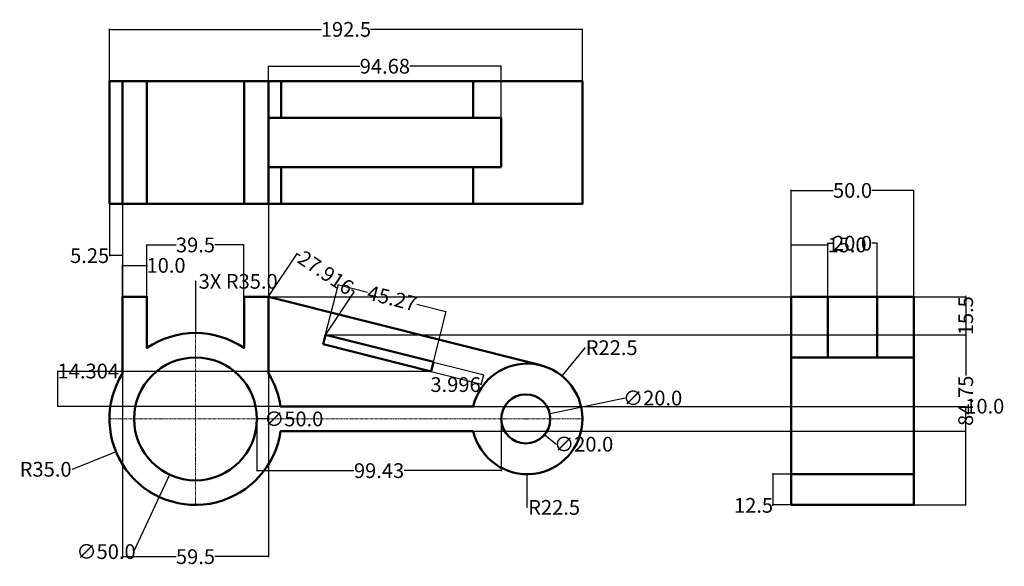
# Model space of a CAD drawing. Units: millimetres. Extents: x -7 to 393, y 19 to 241.
import ezdxf

# ---------------------------------------------------------------- set-up
doc = ezdxf.new("R2010")
doc.units = ezdxf.units.MM
doc.header["$MEASUREMENT"] = 0
doc.linetypes.add('CENTER', pattern=[2, 1.25, -0.25, 0.25, -0.25])
for name, color, linetype, lineweight in [('M-CNTR', 4, 'CENTER', 18), ('M-DIMS', 2, 'Continuous', 25), ('M-OUTL', 7, 'Continuous', 50)]:
    doc.layers.add(name, color=color, linetype=linetype, lineweight=lineweight)
doc.styles.get("Standard").update_dxf_attribs({"font": 'arial.ttf'})
doc.dimstyles.get("Standard").update_dxf_attribs({"dimtxt": 6, "dimasz": 0.18, "dimexe": 0.18, "dimexo": 0.0625, "dimgap": 0.09, "dimtad": 0, "dimtoh": 1, "dimdec": 1, "dimzin": 0, "dimdsep": 46, "dimtxsty": 'Standard', "dimcen": 0.09, "dimadec": 0, "dimazin": 0, "dimtfac": 1, "dimtdec": 1, "dimtofl": 0, "dimtmove": 0, "dimatfit": 3, "dimfxl": 1, "dimtolj": 1, "dimtzin": 0, "dimarcsym": 0})

# ---------------------------------------------------------------- blocks, each defined once
blk = doc.blocks.new('*D1')
at = {"layer": 'Defpoints', "color": 0, "transparency": 16777216}
for p in [(356.5, 171.5), (306.5, 128.25), (356.5, 128.25)]:
    blk.add_point(p, dxfattribs=at)
at = {"layer": 'M-DIMS', "color": 0, "lineweight": -2, "transparency": 16777216}
for p, q in [((306.5, 128.31), (306.5, 171.68)), ((306.68, 171.5), (323.63, 171.5)), ((356.32, 171.5), (339.37, 171.5)), ((356.5, 128.31), (356.5, 171.68))]:
    blk.add_line(p, q, dxfattribs=at)
at = {"layer": 'M-DIMS', "color": 0, "transparency": 16777216}
for points in [[(306.68, 171.53), (306.68, 171.47), (306.5, 171.5)], [(356.32, 171.53), (356.32, 171.47), (356.5, 171.5)]]:
    blk.add_solid(points, dxfattribs=at)
at = {"layer": 'M-DIMS', "color": 0, "transparency": 16777216, "insert": (331.5, 171.5), "char_height": 6, "attachment_point": 5}
blk.add_mtext('\\A1;50.0', dxfattribs=at)
blk = doc.blocks.new('*D2')
at = {"layer": 'Defpoints', "color": 0, "transparency": 16777216}
for p in [(341.5, 150), (321.5, 128.25), (341.5, 128.25)]:
    blk.add_point(p, dxfattribs=at)
at = {"layer": 'M-DIMS', "color": 0, "lineweight": -2, "transparency": 16777216}
for p, q in [((321.5, 128.31), (321.5, 150.18)), ((321.68, 150), (323.58, 150)), ((341.32, 150), (339.42, 150)), ((341.5, 128.31), (341.5, 150.18))]:
    blk.add_line(p, q, dxfattribs=at)
at = {"layer": 'M-DIMS', "color": 0, "transparency": 16777216}
for points in [[(321.68, 150.03), (321.68, 149.97), (321.5, 150)], [(341.32, 150.03), (341.32, 149.97), (341.5, 150)]]:
    blk.add_solid(points, dxfattribs=at)
at = {"layer": 'M-DIMS', "color": 0, "transparency": 16777216, "insert": (331.5, 150), "char_height": 6, "attachment_point": 5}
blk.add_mtext('\\A1;20.0', dxfattribs=at)
blk = doc.blocks.new('*D3')
at = {"layer": 'Defpoints', "color": 0, "transparency": 16777216}
for p in [(306.5, 56), (299, 43.5), (306.5, 43.5)]:
    blk.add_point(p, dxfattribs=at)
at = {"layer": 'M-DIMS', "color": 0, "lineweight": -2, "transparency": 16777216}
for p, q in [((306.44, 56), (298.82, 56)), ((299, 55.82), (299, 43.68)), ((306.44, 43.5), (298.82, 43.5)), ((299, 43.32), (298.82, 43.32)), ((299, 43.5), (299, 43.32))]:
    blk.add_line(p, q, dxfattribs=at)
at = {"layer": 'M-DIMS', "color": 0, "transparency": 16777216}
for points in [[(298.97, 55.82), (299.03, 55.82), (299, 56)], [(298.97, 43.68), (299.03, 43.68), (299, 43.5)]]:
    blk.add_solid(points, dxfattribs=at)
at = {"layer": 'M-DIMS', "color": 0, "transparency": 16777216, "insert": (291.2, 43.32), "char_height": 6, "attachment_point": 5}
blk.add_mtext('\\A1;12.5', dxfattribs=at)
blk = doc.blocks.new('*D4')
at = {"layer": 'Defpoints', "color": 0, "transparency": 16777216}
for p in [(213.21, 96), (199.07, 78.5)]:
    blk.add_point(p, dxfattribs=at)
at = {"layer": 'M-DIMS', "color": 0, "lineweight": -2, "transparency": 16777216}
for p, q in [((222.5, 107.5), (213.32, 96.14)), ((222.68, 107.5), (222.5, 107.5)), ((198.98, 78.5), (199.16, 78.5)), ((199.07, 78.41), (199.07, 78.59))]:
    blk.add_line(p, q, dxfattribs=at)
at = {"layer": 'M-DIMS', "color": 0, "transparency": 16777216}
blk.add_solid([(213.3, 96.16), (213.35, 96.12), (213.21, 96)], dxfattribs=at)
at = {"layer": 'M-DIMS', "color": 0, "transparency": 16777216, "insert": (233.46, 107.5), "char_height": 6, "attachment_point": 5}
blk.add_mtext('\\A1;R22.5', dxfattribs=at)
blk = doc.blocks.new('*D5')
at = {"layer": 'Defpoints', "color": 0, "transparency": 16777216}
for p in [(208.29, 80.55), (188.71, 76.45)]:
    blk.add_point(p, dxfattribs=at)
at = {"layer": 'M-DIMS', "color": 0, "lineweight": -2, "transparency": 16777216}
for p, q in [((239, 87), (208.46, 80.59)), ((198.41, 78.5), (198.59, 78.5)), ((198.5, 78.41), (198.5, 78.59))]:
    blk.add_line(p, q, dxfattribs=at)
at = {"layer": 'M-DIMS', "color": 0, "transparency": 16777216}
blk.add_solid([(208.46, 80.62), (208.47, 80.56), (208.29, 80.55)], dxfattribs=at)
at = {"layer": 'M-DIMS', "color": 0, "transparency": 16777216, "insert": (250.14, 87), "char_height": 6, "attachment_point": 5}
blk.add_mtext('\\A1;∅20.0', dxfattribs=at)
blk = doc.blocks.new('*D6')
at = {"layer": 'Defpoints', "color": 0, "transparency": 16777216}
for p in [(44.32, 141), (34.32, 128.25), (44.32, 128.25)]:
    blk.add_point(p, dxfattribs=at)
at = {"layer": 'M-DIMS', "color": 0, "lineweight": -2, "transparency": 16777216}
for p, q in [((34.32, 128.31), (34.32, 141.18)), ((34.5, 141), (44.14, 141)), ((44.32, 128.31), (44.32, 141.18)), ((44.32, 141), (44.5, 141))]:
    blk.add_line(p, q, dxfattribs=at)
at = {"layer": 'M-DIMS', "color": 0, "transparency": 16777216}
for points in [[(34.5, 141.03), (34.5, 140.97), (34.32, 141)], [(44.14, 141.03), (44.14, 140.97), (44.32, 141)]]:
    blk.add_solid(points, dxfattribs=at)
at = {"layer": 'M-DIMS', "color": 0, "transparency": 16777216, "insert": (52.09, 141), "char_height": 6, "attachment_point": 5}
blk.add_mtext('\\A1;10.0', dxfattribs=at)
blk = doc.blocks.new('*D7')
at = {"layer": 'Defpoints', "color": 0, "transparency": 16777216}
for p in [(64.07, 78.5), (31.68, 65.24)]:
    blk.add_point(p, dxfattribs=at)
at = {"layer": 'M-DIMS', "color": 0, "lineweight": -2, "transparency": 16777216}
for p, q in [((63.98, 78.5), (64.16, 78.5)), ((64.07, 78.41), (64.07, 78.59)), ((14, 58), (31.51, 65.17)), ((13.82, 58), (14, 58))]:
    blk.add_line(p, q, dxfattribs=at)
at = {"layer": 'M-DIMS', "color": 0, "transparency": 16777216}
blk.add_solid([(31.5, 65.2), (31.53, 65.14), (31.68, 65.24)], dxfattribs=at)
at = {"layer": 'M-DIMS', "color": 0, "transparency": 16777216, "insert": (3.08, 58), "char_height": 6, "attachment_point": 5}
blk.add_mtext('\\A1;R35.0', dxfattribs=at)
blk = doc.blocks.new('*D8')
at = {"layer": 'Defpoints', "color": 0, "transparency": 16777216}
for p in [(74.6, 101.18), (53.54, 55.82)]:
    blk.add_point(p, dxfattribs=at)
at = {"layer": 'M-DIMS', "color": 0, "lineweight": -2, "transparency": 16777216}
for p, q in [((63.98, 78.5), (64.16, 78.5)), ((64.07, 78.41), (64.07, 78.59)), ((39, 24.5), (53.47, 55.66)), ((38.82, 24.5), (39, 24.5))]:
    blk.add_line(p, q, dxfattribs=at)
at = {"layer": 'M-DIMS', "color": 0, "transparency": 16777216}
blk.add_solid([(53.44, 55.67), (53.5, 55.65), (53.54, 55.82)], dxfattribs=at)
at = {"layer": 'M-DIMS', "color": 0, "transparency": 16777216, "insert": (27.68, 24.5), "char_height": 6, "attachment_point": 5}
blk.add_mtext('\\A1;∅50.0', dxfattribs=at)
blk = doc.blocks.new('*D9')
at = {"layer": 'Defpoints', "color": 0, "transparency": 16777216}
for p in [(221.57, 237.05), (29.07, 216), (221.57, 216)]:
    blk.add_point(p, dxfattribs=at)
at = {"layer": 'M-DIMS', "color": 0, "lineweight": -2, "transparency": 16777216}
for p, q in [((29.07, 216.06), (29.07, 237.23)), ((29.25, 237.05), (115.37, 237.05)), ((221.39, 237.05), (135.28, 237.05)), ((221.57, 216.06), (221.57, 237.23))]:
    blk.add_line(p, q, dxfattribs=at)
at = {"layer": 'M-DIMS', "color": 0, "transparency": 16777216}
for points in [[(29.25, 237.08), (29.25, 237.02), (29.07, 237.05)], [(221.39, 237.08), (221.39, 237.02), (221.57, 237.05)]]:
    blk.add_solid(points, dxfattribs=at)
at = {"layer": 'M-DIMS', "color": 0, "transparency": 16777216, "insert": (125.32, 237.05), "char_height": 6, "attachment_point": 5}
blk.add_mtext('\\A1;192.5', dxfattribs=at)
blk = doc.blocks.new('*D10')
at = {"layer": 'Defpoints', "color": 0, "transparency": 16777216}
for p in [(356.5, 128.25), (377.55, 128.25), (356.5, 43.5)]:
    blk.add_point(p, dxfattribs=at)
at = {"layer": 'M-DIMS', "color": 0, "lineweight": -2, "transparency": 16777216}
for p, q in [((356.56, 128.25), (377.73, 128.25)), ((377.55, 128.07), (377.55, 96.12)), ((377.55, 43.68), (377.55, 75.63)), ((356.56, 43.5), (377.73, 43.5))]:
    blk.add_line(p, q, dxfattribs=at)
at = {"layer": 'M-DIMS', "color": 0, "transparency": 16777216}
for points in [[(377.52, 128.07), (377.58, 128.07), (377.55, 128.25)], [(377.52, 43.68), (377.58, 43.68), (377.55, 43.5)]]:
    blk.add_solid(points, dxfattribs=at)
at = {"layer": 'M-DIMS', "color": 0, "transparency": 16777216, "insert": (377.55, 85.87), "char_height": 6, "attachment_point": 5, "rotation": 90}
blk.add_mtext('\\A1;84.75', dxfattribs=at)
blk = doc.blocks.new('*D11')
at = {"layer": 'Defpoints', "color": 0, "transparency": 16777216}
for p in [(89.07, 78.5), (188.5, 78.5), (89.07, 57.45)]:
    blk.add_point(p, dxfattribs=at)
at = {"layer": 'M-DIMS', "color": 0, "lineweight": -2, "transparency": 16777216}
for p, q in [((89.07, 78.44), (89.07, 57.27)), ((188.5, 78.44), (188.5, 57.27)), ((89.25, 57.45), (128.57, 57.45)), ((188.32, 57.45), (149, 57.45))]:
    blk.add_line(p, q, dxfattribs=at)
at = {"layer": 'M-DIMS', "color": 0, "transparency": 16777216}
for points in [[(89.25, 57.48), (89.25, 57.42), (89.07, 57.45)], [(188.32, 57.48), (188.32, 57.42), (188.5, 57.45)]]:
    blk.add_solid(points, dxfattribs=at)
at = {"layer": 'M-DIMS', "color": 0, "transparency": 16777216, "insert": (138.79, 57.45), "char_height": 6, "attachment_point": 5}
blk.add_mtext('\\A1;99.43', dxfattribs=at)
blk = doc.blocks.new('*D12')
at = {"layer": 'Defpoints', "color": 0, "transparency": 16777216}
for p in [(98.712775, 83.5), (377.55, 83.5), (98.712775, 73.5)]:
    blk.add_point(p, dxfattribs=at)
at = {"layer": 'M-DIMS', "color": 0, "lineweight": -2, "transparency": 16777216}
for p, q in [((98.775275, 83.5), (377.73, 83.5)), ((377.55, 83.5), (377.55, 83.68)), ((377.55, 83.68), (377.73, 83.68)), ((377.55, 73.68), (377.55, 83.32)), ((98.775275, 73.5), (377.73, 73.5))]:
    blk.add_line(p, q, dxfattribs=at)
at = {"layer": 'M-DIMS', "color": 0, "transparency": 16777216}
for points in [[(377.52, 83.32), (377.58, 83.32), (377.55, 83.5)], [(377.52, 73.68), (377.58, 73.68), (377.55, 73.5)]]:
    blk.add_solid(points, dxfattribs=at)
at = {"layer": 'M-DIMS', "color": 0, "transparency": 16777216, "insert": (385.32, 83.68), "char_height": 6, "attachment_point": 5}
blk.add_mtext('\\A1;10.0', dxfattribs=at)
blk = doc.blocks.new('*D13')
at = {"layer": 'Defpoints', "color": 0, "transparency": 16777216}
for p in [(34.32, 166), (93.82, 166), (93.82, 22.45)]:
    blk.add_point(p, dxfattribs=at)
at = {"layer": 'M-DIMS', "color": 0, "lineweight": -2, "transparency": 16777216}
for p, q in [((34.32, 165.94), (34.32, 22.27)), ((93.82, 165.94), (93.82, 22.27)), ((34.5, 22.45), (56.17, 22.45)), ((93.64, 22.45), (71.98, 22.45))]:
    blk.add_line(p, q, dxfattribs=at)
at = {"layer": 'M-DIMS', "color": 0, "transparency": 16777216}
for points in [[(34.5, 22.48), (34.5, 22.42), (34.32, 22.45)], [(93.64, 22.48), (93.64, 22.42), (93.82, 22.45)]]:
    blk.add_solid(points, dxfattribs=at)
at = {"layer": 'M-DIMS', "color": 0, "transparency": 16777216, "insert": (64.07, 22.45), "char_height": 6, "attachment_point": 5}
blk.add_mtext('\\A1;59.5', dxfattribs=at)
blk = doc.blocks.new('*D14')
at = {"layer": 'Defpoints', "color": 0, "transparency": 16777216}
for p in [(166.08, 122.09), (117.04, 112.75), (160.93, 101.68)]:
    blk.add_point(p, dxfattribs=at)
at = {"layer": 'M-DIMS', "color": 0, "lineweight": -2, "transparency": 16777216}
for p, q in [((117.05, 112.81), (122.23, 133.34)), ((122.36, 133.12), (134.11, 130.15)), ((165.91, 122.13), (154.16, 125.1)), ((160.95, 101.74), (166.13, 122.26))]:
    blk.add_line(p, q, dxfattribs=at)
at = {"layer": 'M-DIMS', "color": 0, "transparency": 16777216}
for points in [[(122.37, 133.15), (122.35, 133.09), (122.19, 133.16)], [(165.92, 122.16), (165.9, 122.1), (166.08, 122.09)]]:
    blk.add_solid(points, dxfattribs=at)
at = {"layer": 'M-DIMS', "color": 0, "transparency": 16777216, "insert": (144.13, 127.63), "char_height": 6, "attachment_point": 5, "rotation": 345.8445}
blk.add_mtext('\\A1;45.27', dxfattribs=at)
blk = doc.blocks.new('*D15')
at = {"layer": 'Defpoints', "color": 0, "transparency": 16777216}
for p in [(160.93, 101.68), (159.96, 97.8), (180.37, 92.66)]:
    blk.add_point(p, dxfattribs=at)
at = {"layer": 'M-DIMS', "color": 0, "lineweight": -2, "transparency": 16777216}
for p, q in [((160.99, 101.66), (181.52, 96.49)), ((160.02, 97.79), (180.54, 92.61)), ((181.3, 96.36), (180.41, 92.83)), ((180.32, 92.48), (180.14, 92.48)), ((180.37, 92.66), (180.32, 92.48))]:
    blk.add_line(p, q, dxfattribs=at)
at = {"layer": 'M-DIMS', "color": 0, "transparency": 16777216}
for points in [[(181.27, 96.36), (181.33, 96.35), (181.35, 96.53)], [(180.38, 92.84), (180.44, 92.82), (180.37, 92.66)]]:
    blk.add_solid(points, dxfattribs=at)
at = {"layer": 'M-DIMS', "color": 0, "transparency": 16777216, "insert": (169.93, 92.48), "char_height": 6, "attachment_point": 5}
blk.add_mtext('\\A1;3.996', dxfattribs=at)
blk = doc.blocks.new('*D16')
at = {"layer": 'Defpoints', "color": 0, "transparency": 16777216}
for p in [(93.82, 128.25), (117.04, 112.75), (377.55, 112.75)]:
    blk.add_point(p, dxfattribs=at)
at = {"layer": 'M-DIMS', "color": 0, "lineweight": -2, "transparency": 16777216}
for p, q in [((93.88, 128.25), (377.73, 128.25)), ((377.55, 128.43), (377.55, 128.61)), ((117.1, 112.75), (377.73, 112.75)), ((377.55, 112.57), (377.55, 112.39))]:
    blk.add_line(p, q, dxfattribs=at)
at = {"layer": 'M-DIMS', "color": 0, "transparency": 16777216}
for points in [[(377.52, 128.43), (377.58, 128.43), (377.55, 128.25)], [(377.52, 112.57), (377.58, 112.57), (377.55, 112.75)]]:
    blk.add_solid(points, dxfattribs=at)
at = {"layer": 'M-DIMS', "color": 0, "transparency": 16777216, "insert": (377.55, 120.5), "char_height": 6, "attachment_point": 5, "rotation": 90}
blk.add_mtext('\\A1;15.5', dxfattribs=at)
blk = doc.blocks.new('*D17')
at = {"layer": 'Defpoints', "color": 0, "transparency": 16777216}
for p in [(188.5, 222.05), (93.82, 201), (188.5, 201)]:
    blk.add_point(p, dxfattribs=at)
at = {"layer": 'M-DIMS', "color": 0, "lineweight": -2, "transparency": 16777216}
for p, q in [((93.82, 201.06), (93.82, 222.23)), ((94, 222.05), (130.94, 222.05)), ((188.32, 222.05), (151.38, 222.05)), ((188.5, 201.06), (188.5, 222.23))]:
    blk.add_line(p, q, dxfattribs=at)
at = {"layer": 'M-DIMS', "color": 0, "transparency": 16777216}
for points in [[(94, 222.08), (94, 222.02), (93.82, 222.05)], [(188.32, 222.08), (188.32, 222.02), (188.5, 222.05)]]:
    blk.add_solid(points, dxfattribs=at)
at = {"layer": 'M-DIMS', "color": 0, "transparency": 16777216, "insert": (141.16, 222.05), "char_height": 6, "attachment_point": 5}
blk.add_mtext('\\A1;94.68', dxfattribs=at)
blk = doc.blocks.new('*D18')
at = {"layer": 'Defpoints', "color": 0, "transparency": 16777216}
for p in [(93.82, 128.25), (128.73, 130.26), (117.04, 112.75)]:
    blk.add_point(p, dxfattribs=at)
at = {"layer": 'M-DIMS', "color": 0, "lineweight": -2, "transparency": 16777216}
for p, q in [((93.86, 128.3), (105.61, 145.91)), ((105.66, 145.66), (106.64, 145)), ((117.07, 112.8), (128.83, 130.41)), ((128.58, 130.36), (127.59, 131.01))]:
    blk.add_line(p, q, dxfattribs=at)
at = {"layer": 'M-DIMS', "color": 0, "transparency": 16777216}
for points in [[(105.68, 145.68), (105.64, 145.63), (105.51, 145.76)], [(128.59, 130.38), (128.56, 130.33), (128.73, 130.26)]]:
    blk.add_solid(points, dxfattribs=at)
at = {"layer": 'M-DIMS', "color": 0, "transparency": 16777216, "insert": (117.12, 138.01), "char_height": 6, "attachment_point": 5, "rotation": 326.2729}
blk.add_mtext('\\A1;27.916', dxfattribs=at)
blk = doc.blocks.new('*D19')
at = {"layer": 'Defpoints', "color": 0, "transparency": 16777216}
for p in [(29.07, 166), (34.32, 166), (29.07, 144.95)]:
    blk.add_point(p, dxfattribs=at)
at = {"layer": 'M-DIMS', "color": 0, "lineweight": -2, "transparency": 16777216}
for p, q in [((29.07, 165.94), (29.07, 144.77)), ((34.32, 165.94), (34.32, 144.77)), ((29.07, 144.95), (28.89, 144.95)), ((34.14, 144.95), (29.25, 144.95))]:
    blk.add_line(p, q, dxfattribs=at)
at = {"layer": 'M-DIMS', "color": 0, "transparency": 16777216}
for points in [[(29.25, 144.98), (29.25, 144.92), (29.07, 144.95)], [(34.14, 144.98), (34.14, 144.92), (34.32, 144.95)]]:
    blk.add_solid(points, dxfattribs=at)
at = {"layer": 'M-DIMS', "color": 0, "transparency": 16777216, "insert": (20.99, 144.95), "char_height": 6, "attachment_point": 5}
blk.add_mtext('\\A1;5.25', dxfattribs=at)
blk = doc.blocks.new('*D20')
at = {"layer": 'Defpoints', "color": 0, "transparency": 16777216}
for p in [(321.5, 149.3), (306.5, 128.25), (321.5, 128.25)]:
    blk.add_point(p, dxfattribs=at)
at = {"layer": 'M-DIMS', "color": 0, "lineweight": -2, "transparency": 16777216}
for p, q in [((306.5, 128.3125), (306.5, 149.48)), ((306.68, 149.3), (321.32, 149.3)), ((321.5, 128.3125), (321.5, 149.48)), ((321.5, 149.3), (321.68, 149.3))]:
    blk.add_line(p, q, dxfattribs=at)
at = {"layer": 'M-DIMS', "color": 0, "transparency": 16777216}
for points in [[(306.68, 149.33), (306.68, 149.27), (306.5, 149.3)], [(321.32, 149.33), (321.32, 149.27), (321.5, 149.3)]]:
    blk.add_solid(points, dxfattribs=at)
at = {"layer": 'M-DIMS', "color": 0, "transparency": 16777216, "insert": (329.27, 149.3), "char_height": 6, "attachment_point": 5}
blk.add_mtext('\\A1;15.0', dxfattribs=at)
blk = doc.blocks.new('*D21')
at = {"layer": 'Defpoints', "color": 0, "transparency": 16777216}
for p in [(8.02, 97.8), (159.96, 97.8), (177.13, 83.5)]:
    blk.add_point(p, dxfattribs=at)
at = {"layer": 'M-DIMS', "color": 0, "lineweight": -2, "transparency": 16777216}
for p, q in [((159.89, 97.8), (7.84, 97.8)), ((8.02, 97.8), (8.02, 97.98)), ((8.02, 97.98), (8.2, 97.98)), ((8.02, 83.68), (8.02, 97.62)), ((177.07, 83.5), (7.84, 83.5))]:
    blk.add_line(p, q, dxfattribs=at)
at = {"layer": 'M-DIMS', "color": 0, "transparency": 16777216}
for points in [[(7.99, 97.62), (8.05, 97.62), (8.02, 97.8)], [(7.99, 83.68), (8.05, 83.68), (8.02, 83.5)]]:
    blk.add_solid(points, dxfattribs=at)
at = {"layer": 'M-DIMS', "color": 0, "transparency": 16777216, "insert": (20.45, 97.98), "char_height": 6, "attachment_point": 5}
blk.add_mtext('\\A1;14.304', dxfattribs=at)
blk = doc.blocks.new('*D22')
at = {"layer": 'Defpoints', "color": 0, "transparency": 16777216}
for p in [(83.82, 149.3), (44.32, 128.25), (83.82, 128.25)]:
    blk.add_point(p, dxfattribs=at)
at = {"layer": 'M-DIMS', "color": 0, "lineweight": -2, "transparency": 16777216}
for p, q in [((44.32, 128.31), (44.32, 149.48)), ((44.5, 149.3), (56.17, 149.3)), ((83.64, 149.3), (71.97, 149.3)), ((83.82, 128.31), (83.82, 149.48))]:
    blk.add_line(p, q, dxfattribs=at)
at = {"layer": 'M-DIMS', "color": 0, "transparency": 16777216}
for points in [[(44.5, 149.33), (44.5, 149.27), (44.32, 149.3)], [(83.64, 149.33), (83.64, 149.27), (83.82, 149.3)]]:
    blk.add_solid(points, dxfattribs=at)
at = {"layer": 'M-DIMS', "color": 0, "transparency": 16777216, "insert": (64.07, 149.3), "char_height": 6, "attachment_point": 5}
blk.add_mtext('\\A1;39.5', dxfattribs=at)
blk = doc.blocks.new('*D23')
at = {"layer": 'Defpoints', "color": 0, "transparency": 16777216}
for p in [(64.07, 113.5), (64.07, 78.5)]:
    blk.add_point(p, dxfattribs=at)
at = {"layer": 'M-DIMS', "color": 0, "lineweight": -2, "transparency": 16777216}
for p, q in [((64.25, 134.5), (64.07, 134.5)), ((64.07, 134.5), (64.07, 113.68)), ((63.98, 78.5), (64.16, 78.5)), ((64.07, 78.41), (64.07, 78.59))]:
    blk.add_line(p, q, dxfattribs=at)
at = {"layer": 'M-DIMS', "color": 0, "transparency": 16777216}
blk.add_solid([(64.04, 113.68), (64.1, 113.68), (64.07, 113.5)], dxfattribs=at)
at = {"layer": 'M-DIMS', "color": 0, "transparency": 16777216, "insert": (81.44, 134.5), "char_height": 6, "attachment_point": 5}
blk.add_mtext('\\A1;3X R35.0', dxfattribs=at)
blk = doc.blocks.new('*D24')
at = {"layer": 'Defpoints', "color": 0, "transparency": 16777216}
for p in [(39.07, 78.5), (89.07, 78.5)]:
    blk.add_point(p, dxfattribs=at)
at = {"layer": 'M-DIMS', "color": 0, "lineweight": -2, "transparency": 16777216}
for p, q in [((63.98, 78.5), (64.16, 78.5)), ((64.07, 78.41), (64.07, 78.59)), ((92.94, 78.5), (89.25, 78.5))]:
    blk.add_line(p, q, dxfattribs=at)
at = {"layer": 'M-DIMS', "color": 0, "transparency": 16777216}
blk.add_solid([(89.25, 78.53), (89.25, 78.47), (89.07, 78.5)], dxfattribs=at)
at = {"layer": 'M-DIMS', "color": 0, "transparency": 16777216, "insert": (104.07, 78.5), "char_height": 6, "attachment_point": 5}
blk.add_mtext('\\A1;∅50.0', dxfattribs=at)
blk = doc.blocks.new('*D25')
at = {"layer": 'Defpoints', "color": 0, "transparency": 16777216}
for p in [(199.07, 78.5), (199.07, 56)]:
    blk.add_point(p, dxfattribs=at)
at = {"layer": 'M-DIMS', "color": 0, "lineweight": -2, "transparency": 16777216}
for p, q in [((198.98, 78.5), (199.16, 78.5)), ((199.07, 78.41), (199.07, 78.59)), ((199.07, 42.5), (199.07, 55.82)), ((199.25, 42.5), (199.07, 42.5))]:
    blk.add_line(p, q, dxfattribs=at)
at = {"layer": 'M-DIMS', "color": 0, "transparency": 16777216}
blk.add_solid([(199.1, 55.82), (199.04, 55.82), (199.07, 56)], dxfattribs=at)
at = {"layer": 'M-DIMS', "color": 0, "transparency": 16777216, "insert": (210.03, 42.5), "char_height": 6, "attachment_point": 5}
blk.add_mtext('\\A1;R22.5', dxfattribs=at)
blk = doc.blocks.new('*D26')
at = {"layer": 'Defpoints', "color": 0, "transparency": 16777216}
for p in [(190.84, 84.93), (206.16, 72.07)]:
    blk.add_point(p, dxfattribs=at)
at = {"layer": 'M-DIMS', "color": 0, "lineweight": -2, "transparency": 16777216}
for p, q in [((198.41, 78.5), (198.59, 78.5)), ((198.5, 78.41), (198.5, 78.59)), ((210.75, 68.21), (206.3, 71.95)), ((210.93, 68.21), (210.75, 68.21))]:
    blk.add_line(p, q, dxfattribs=at)
at = {"layer": 'M-DIMS', "color": 0, "transparency": 16777216}
blk.add_solid([(206.32, 71.98), (206.28, 71.93), (206.16, 72.07)], dxfattribs=at)
at = {"layer": 'M-DIMS', "color": 0, "transparency": 16777216, "insert": (222.07, 68.21), "char_height": 6, "attachment_point": 5}
blk.add_mtext('\\A1;∅20.0', dxfattribs=at)

msp = doc.modelspace()

# ---------------------------------------------------------------- linework, layer by layer
at = {"layer": 'M-CNTR'}
for p, q in [((64.0718, 43.5), (64.0718, 128.25)), ((29.0718, 81), (29.1612, 81)), ((221.4324, 81), (221.5718, 81)), ((29.0718, 78.5), (221.5718, 78.5)), ((29.0718, 76), (29.1612, 76)), ((221.4324, 76), (221.5718, 76))]:
    msp.add_line(p, q, dxfattribs=at)
at = {"layer": 'M-OUTL'}
for p, q in [((34.3218, 166), (34.3218, 216)), ((44.3218, 166), (44.3218, 216)), ((83.8218, 166), (83.8218, 216)), ((93.8218, 166), (93.8218, 216)), ((98.9824, 201), (98.9824, 216)), ((177.1318, 216), (177.1318, 201)), ((188.5, 191), (188.5318, 191)), ((98.9824, 166), (98.9824, 181)), ((177.1318, 181), (177.1318, 166)), ((321.5, 103.5), (321.5, 128.25)), ((341.5, 128.25), (341.5, 103.5)), ((306.5, 103.5), (356.5, 103.5)), ((306.5, 56), (356.5, 56))]:
    msp.add_line(p, q, dxfattribs=at)
for points in [[(29.0718, 166), (29.0718, 216), (221.5718, 216), (221.5718, 166)], [(306.5, 43.5), (356.5, 43.5), (356.5, 128.25), (306.5, 128.25)]]:
    msp.add_lwpolyline(points, close=True, dxfattribs=at)
for points in [[(93.8218, 201), (177.1318, 201), (188.5, 201), (188.5, 181)], [(93.8218, 181), (177.1318, 181), (188.5318, 181)], [(159.9561, 97.8004), (160.9344, 101.679), (117.0395, 112.7498), (116.0623, 108.8753), (159.9571, 97.8044)]]:
    msp.add_lwpolyline(points, dxfattribs=at)
for points in [[(177.1343, 73.5), (98.7128, 73.5, -1.23022683), (34.3218, 96.9374), (34.3218, 128.25), (44.3218, 128.25), (44.3218, 107.3953, -0.30909949), (83.8218, 107.3953), (83.8218, 128.25), (93.8218, 128.25), (204.5742, 100.3168)], [(177.1343, 73.5, 8.88748219), (177.1343, 83.5), (98.7128, 83.5, 0.10323023), (93.8218, 96.9374), (93.8218, 128.25)]]:
    msp.add_lwpolyline(points, format="xyb", dxfattribs=at)
for centre, radius in [((64.0718, 78.5), 25), ((198.5, 78.5), 10)]:
    msp.add_circle(centre, radius, dxfattribs=at)

# ---------------------------------------------------------------- dimensions: what is measured, and where the dimension line sits
at = {"layer": 'M-DIMS'}
for base, p1, p2, override, picture, middle in [((221.5718, 237.05), (29.0718, 216), (221.5718, 216), {"dimdec": 1, "dimlfac": 1, "dimrnd": 0, "dimzin": 0, "dimdsep": 46, "dimlunit": 2}, '*D9', (125.3218, 237.05)), ((188.5, 222.05), (93.8218, 201), (188.5, 201), {"dimdec": 2, "dimlfac": 1, "dimrnd": 0, "dimzin": 0, "dimdsep": 46, "dimlunit": 2}, '*D17', (141.1609, 222.05)), ((356.5, 171.5), (306.5, 128.25), (356.5, 128.25), {"dimclrd": 0, "dimclre": 0, "dimclrt": 0}, '*D1', (331.5, 171.5)), ((93.8218, 22.45), (34.3218, 166), (93.8218, 166), {"dimdec": 1, "dimlfac": 1, "dimrnd": 0, "dimzin": 0, "dimdsep": 46, "dimlunit": 2}, '*D13', (64.0718, 22.45)), ((83.8218, 149.3), (44.3218, 128.25), (83.8218, 128.25), {"dimdec": 1, "dimlfac": 1, "dimrnd": 0, "dimzin": 0, "dimdsep": 46, "dimlunit": 2}, '*D22', (64.0718, 149.3)), ((321.5, 149.3), (306.5, 128.25), (321.5, 128.25), {"dimdec": 1, "dimlfac": 1, "dimrnd": 0, "dimzin": 0, "dimdsep": 46, "dimlunit": 2}, '*D20', (329.27, 149.3)), ((341.5, 150), (321.5, 128.25), (341.5, 128.25), {"dimclrd": 0, "dimclre": 0, "dimclrt": 0}, '*D2', (331.5, 150)), ((44.3218, 141), (34.3218, 128.25), (44.3218, 128.25), {"dimclrd": 0, "dimclre": 0, "dimclrt": 0}, '*D6', (52.0918, 141))]:
    dim = msp.add_linear_dim(base=base, p1=p1, p2=p2, dimstyle='Standard', override=override, dxfattribs=at)
    dim.commit()
    dim.dimension.update_dxf_attribs({"geometry": picture, "text_midpoint": middle})
for base, p1, p2, angle, override, picture, middle in [((29.0718, 144.95), (34.3218, 166), (29.0718, 166), 180, {"dimdec": 2, "dimlfac": 1, "dimrnd": 0, "dimzin": 0, "dimdsep": 46, "dimlunit": 2}, '*D19', (20.9866, 144.95)), ((128.7272, 130.2569), (93.8218, 128.25), (117.0395, 112.7498), 326.272871, {"dimdec": 3, "dimlfac": 1, "dimrnd": 0, "dimzin": 0, "dimdsep": 46, "dimlunit": 2}, '*D18', (117.1184, 138.007)), ((166.0822, 122.0898), (117.0395, 112.7498), (160.9344, 101.679), 345.844489, {"dimdec": 2, "dimlfac": 1, "dimrnd": 0, "dimzin": 0, "dimdsep": 46, "dimlunit": 2}, '*D14', (144.1348, 127.6252)), ((377.55, 112.7498), (93.8218, 128.25), (117.0395, 112.7498), 90, {"dimdec": 1, "dimlfac": 1, "dimrnd": 0, "dimzin": 0, "dimdsep": 46, "dimlunit": 2}, '*D16', (377.55, 120.4999)), ((377.55, 128.25), (356.5, 43.5), (356.5, 128.25), 90, {"dimdec": 2, "dimlfac": 1, "dimrnd": 0, "dimzin": 0, "dimdsep": 46, "dimlunit": 2}, '*D10', (377.55, 85.875)), ((8.0218, 97.8044), (177.1343, 83.5), (159.9571, 97.8044), 90, {"dimdec": 3, "dimlfac": 1, "dimrnd": 0, "dimzin": 0, "dimdsep": 46, "dimlunit": 2}, '*D21', (20.4514, 97.9844)), ((180.368, 92.6566), (160.9344, 101.679), (159.9571, 97.8044), 255.844489, {"dimdec": 3, "dimlfac": 1, "dimrnd": 0, "dimzin": 0, "dimdsep": 46, "dimlunit": 2}, '*D15', (169.9346, 92.482)), ((377.55, 83.5), (98.7128, 73.5), (98.7128, 83.5), 90, {"dimdec": 1, "dimlfac": 1, "dimrnd": 0, "dimzin": 0, "dimdsep": 46, "dimlunit": 2}, '*D12', (385.32, 83.68)), ((89.0718, 57.45), (188.5, 78.5), (89.0718, 78.5), 180, {"dimdec": 2, "dimlfac": 1, "dimrnd": 0, "dimzin": 0, "dimdsep": 46, "dimlunit": 2}, '*D11', (138.7859, 57.45)), ((299, 43.5), (306.5, 56), (306.5, 43.5), 90, {"dimclrd": 0, "dimclre": 0, "dimclrt": 0}, '*D3', (291.1973, 43.32))]:
    dim = msp.add_linear_dim(base=base, p1=p1, p2=p2, angle=angle, dimstyle='Standard', override=override, dxfattribs=at)
    dim.commit()
    dim.dimension.update_dxf_attribs({"geometry": picture, "text_midpoint": middle})
dim = msp.add_radius_dim(center=(64.0718, 78.5), mpoint=(64.072, 113.5), text='3X <>', dimstyle='Standard', override={"dimdec": 1, "dimlfac": 1, "dimrnd": 0, "dimzin": 0, "dimdsep": 46, "dimlunit": 2}, dxfattribs=at)
dim.commit()
dim.dimension.update_dxf_attribs({"geometry": '*D23', "text_midpoint": (81.4397, 134.5), "dimtype": 164})
for center, mpoint, override, picture, middle in [((199.0718, 78.5), (213.2112, 96.0022), {"dimclrd": 0, "dimclre": 0, "dimclrt": 0}, '*D4', (233.4562, 107.5)), ((64.0718, 78.5), (31.6813, 65.2389), {"dimclrd": 0, "dimclre": 0, "dimclrt": 0}, '*D7', (3.0765, 58)), ((199.0718, 78.5), (199.072, 56), {"dimdec": 1, "dimlfac": 1, "dimrnd": 0, "dimzin": 0, "dimdsep": 46, "dimlunit": 2}, '*D25', (210.0284, 42.5))]:
    dim = msp.add_radius_dim(center=center, mpoint=mpoint, dimstyle='Standard', override=override, dxfattribs=at)
    dim.commit()
    dim.dimension.update_dxf_attribs({"geometry": picture, "text_midpoint": middle, "dimtype": 164})
for p1, p2, override, picture, middle in [((74.5997, 101.1752), (53.5439, 55.8248), {"dimclrd": 0, "dimclre": 0, "dimclrt": 0}, '*D8', (27.6836, 24.5)), ((188.7132, 76.446), (208.2868, 80.554), {"dimclrd": 0, "dimclre": 0, "dimclrt": 0}, '*D5', (239, 87)), ((190.8408, 84.9293), (206.1592, 72.0707), {"dimdec": 1, "dimlfac": 1, "dimrnd": 0, "dimzin": 0, "dimdsep": 46, "dimlunit": 2}, '*D26', (222.0711, 68.2131)), ((39.0718, 78.5), (89.0718, 78.5), {"dimdec": 1, "dimlfac": 1, "dimrnd": 0, "dimzin": 0, "dimdsep": 46, "dimlunit": 2}, '*D24', (104.0718, 78.5))]:
    dim = msp.add_diameter_dim_2p(p1=p1, p2=p2, dimstyle='Standard', override=override, dxfattribs=at)
    dim.commit()
    dim.dimension.update_dxf_attribs({"geometry": picture, "text_midpoint": middle, "dimtype": 163})

doc.saveas('drawing.dxf')
